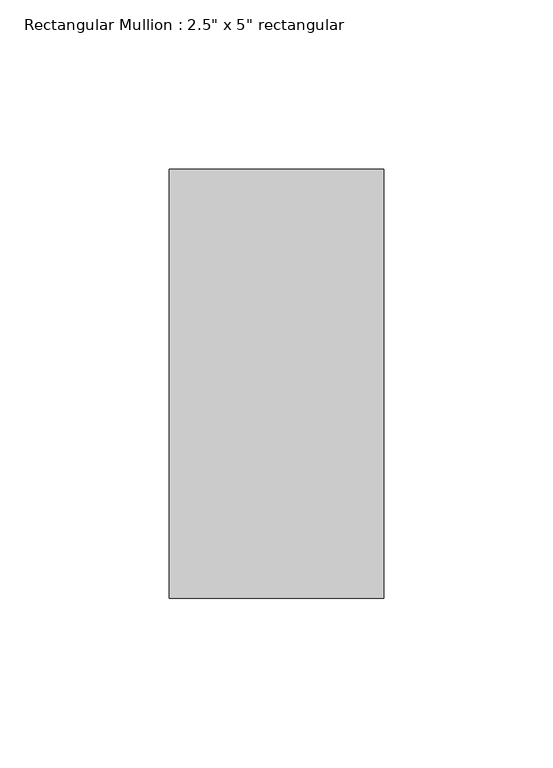
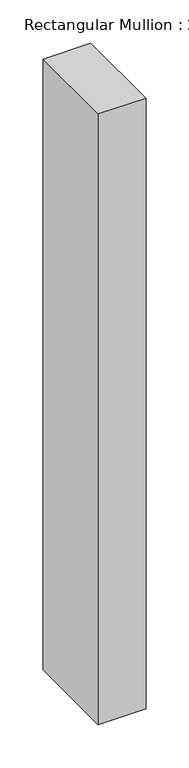
"""IFC4 building model written with IfcOpenShell, lengths in millimetres: member geometry."""

from ifc_helpers import new_model, si_unit, frame, origin, place, context, project, spatial, polyline, outline, extrude, source, transform, mapped, element, save


def member_afcd4490(model_context):
    return source(origin(), model_context, "Body", "SweptSolid", [
        extrude(outline(polyline([(0.0, 63.5), (0.0, -63.5), (-63.5, -63.5), (-63.5, 63.5), (0.0, 63.5)])), frame((0.0, 0.0, -860.4662548), z_axis=(0.0, 0.0, 1.0), x_axis=(1.0, 0.0, 0.0)), (0.0, 0.0, 1.0), 860.4662548),
    ])


if __name__ == "__main__":
    model = new_model("IFC4")
    model_context = context("Model", 3, world=origin())
    ifc_project = project(units=[si_unit("LENGTHUNIT", "METRE", prefix="MILLI")], contexts=[model_context])
    site = spatial("IfcSite", under=ifc_project)
    building = spatial("IfcBuilding", under=site)
    placement = place(None, origin())
    member_shape = member_afcd4490(model_context)
    element("IfcMember", 1, ObjectType="Rectangular Mullion : 2.5\" x 5\" rectangular", at=placement, inside=building, context=model_context, shape_type="MappedRepresentation", body=[
        mapped(member_shape, transform((0.0, 0.0, 0.0), x_axis=(1.0, 0.0, 0.0), y_axis=(0.0, 1.0, 0.0), z_axis=(0.0, 0.0, 1.0))),
    ])
    save(model, "model.ifc")

# Revit data of these elements
# Type "Rectangular Mullion : 2.5\" x 5\" rectangular"
#   built-in parameter 1007304 = 0.416667 (stored number, unit not read)
#   built-in parameter 1007301 = 0.104167 (stored number, unit not read)
#   built-in parameter 1007300 = 0.104167 (stored number, unit not read)
# Element 1 (IfcMember, "Rectangular Mullion : 2.5\" x 5\" rectangular")
#   Materials on its faces: "Aluminum"
# Materials
#   "Aluminum": class "Metal", colour RGB 247 247 247, transparency 0, Description = "Aluminum 6061", Cost = 0
